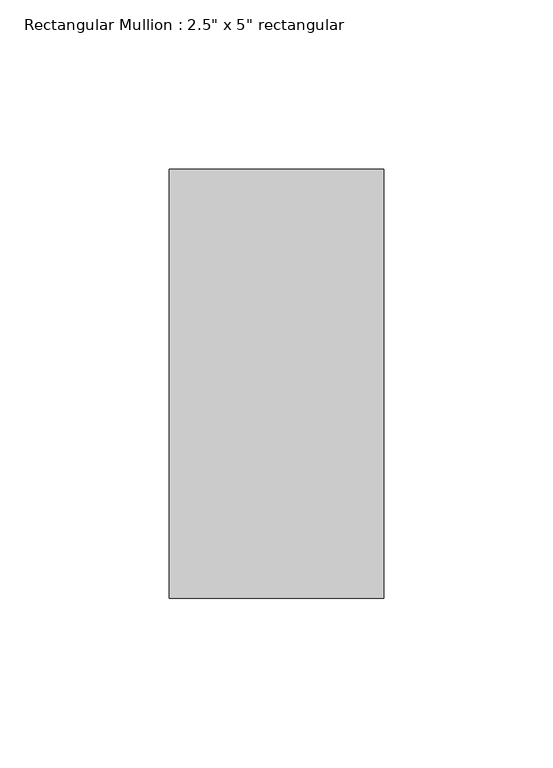
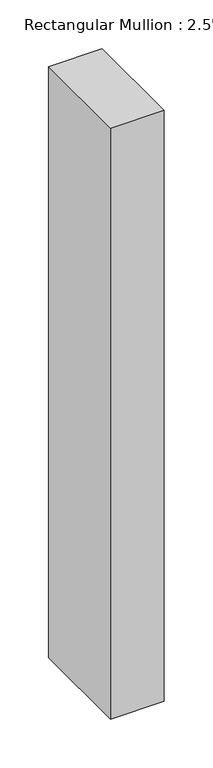
"""IFC4 building model written with IfcOpenShell, lengths in millimetres: member geometry."""

from ifc_helpers import new_model, si_unit, frame, origin, place, context, project, spatial, polyline, outline, extrude, source, transform, mapped, element, save


def member_891d357d(model_context):
    return source(origin(), model_context, "Body", "SweptSolid", [
        extrude(outline(polyline([(0.0, 63.5), (0.0, -63.5), (-63.5, -63.5), (-63.5, 63.5), (0.0, 63.5)])), frame((0.0, 0.0, -740.2112955), z_axis=(0.0, 0.0, 1.0), x_axis=(1.0, 0.0, 0.0)), (0.0, 0.0, 1.0), 740.2112955),
    ])


if __name__ == "__main__":
    model = new_model("IFC4")
    model_context = context("Model", 3, world=origin())
    ifc_project = project(units=[si_unit("LENGTHUNIT", "METRE", prefix="MILLI")], contexts=[model_context])
    site = spatial("IfcSite", under=ifc_project)
    building = spatial("IfcBuilding", under=site)
    placement = place(None, origin())
    member_shape = member_891d357d(model_context)
    element("IfcMember", 1, ObjectType="Rectangular Mullion : 2.5\" x 5\" rectangular", at=placement, inside=building, context=model_context, shape_type="MappedRepresentation", body=[
        mapped(member_shape, transform((0.0, 0.0, 0.0), x_axis=(1.0, 0.0, 0.0), y_axis=(0.0, 1.0, 0.0), z_axis=(0.0, 0.0, 1.0))),
    ])
    save(model, "model.ifc")

# Revit data of these elements
# Type "Rectangular Mullion : 2.5\" x 5\" rectangular"
#   built-in parameter 1007304 = 0.416667 (stored number, unit not read)
#   built-in parameter 1007301 = 0.104167 (stored number, unit not read)
#   built-in parameter 1007300 = 0.104167 (stored number, unit not read)
# Element 1 (IfcMember, "Rectangular Mullion : 2.5\" x 5\" rectangular")
#   Materials on its faces: "Aluminum"
# Materials
#   "Aluminum": class "Metal", colour RGB 247 247 247, transparency 0, Description = "Aluminum 6061", Cost = 0
